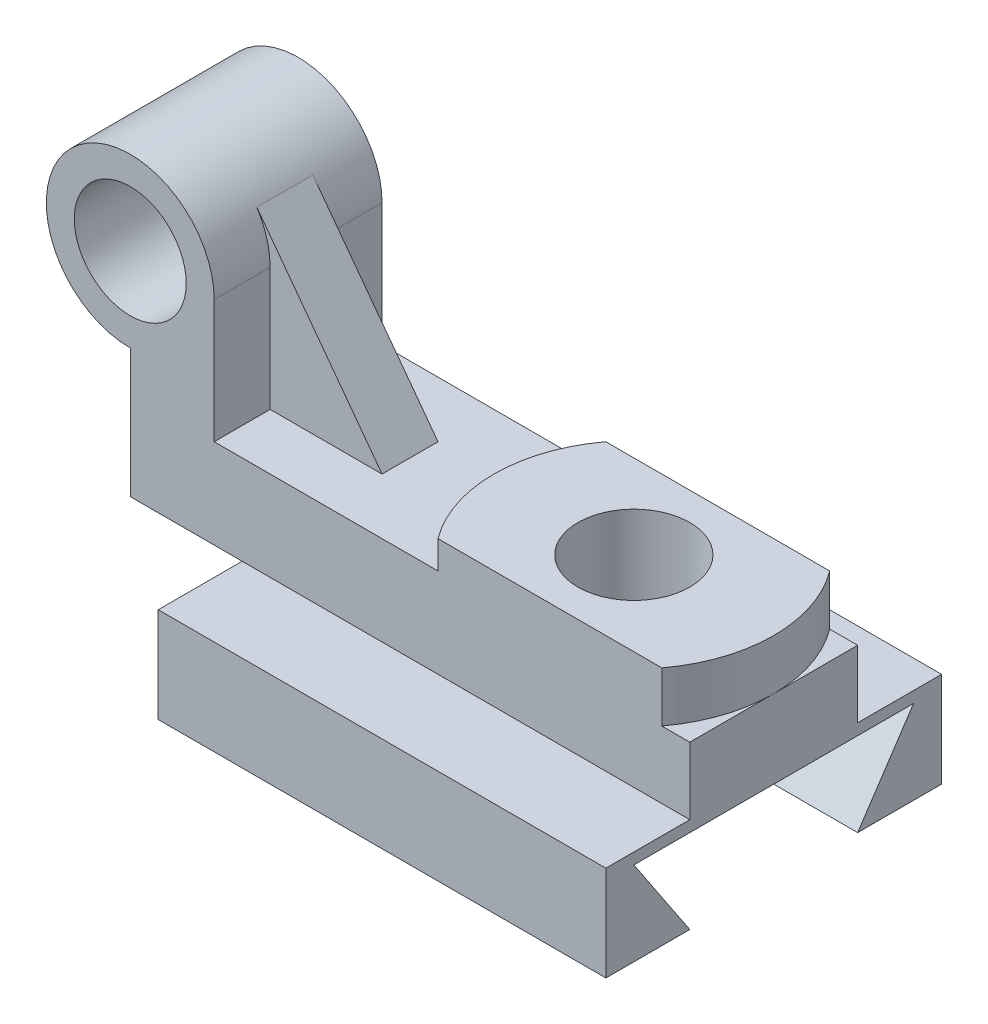
ISO-10303-21;
HEADER;
FILE_DESCRIPTION(('STEP AP214'),'2;1');
FILE_NAME('part.step','',(''),(''),'','','');
FILE_SCHEMA(('AUTOMOTIVE_DESIGN { 1 0 10303 214 1 1 1 1 }'));
ENDSEC;
DATA;
#1=APPLICATION_CONTEXT('core data for automotive mechanical design processes');
#2=APPLICATION_PROTOCOL_DEFINITION('international standard','automotive_design',2000,#1);
#3=PRODUCT_CONTEXT('',#1,'mechanical');
#4=PRODUCT('Part','Part','',(#3));
#5=PRODUCT_RELATED_PRODUCT_CATEGORY('part','',(#4));
#6=PRODUCT_DEFINITION_FORMATION('','',#4);
#7=PRODUCT_DEFINITION_CONTEXT('part definition',#1,'design');
#8=PRODUCT_DEFINITION('design','',#6,#7);
#9=PRODUCT_DEFINITION_SHAPE('','',#8);
#10=(LENGTH_UNIT() NAMED_UNIT(*) SI_UNIT(.MILLI.,.METRE.));
#11=(NAMED_UNIT(*) PLANE_ANGLE_UNIT() SI_UNIT($,.RADIAN.));
#12=(NAMED_UNIT(*) SI_UNIT($,.STERADIAN.) SOLID_ANGLE_UNIT());
#13=UNCERTAINTY_MEASURE_WITH_UNIT(LENGTH_MEASURE(1.E-05),#10,'distance_accuracy_value','');
#14=(GEOMETRIC_REPRESENTATION_CONTEXT(3) GLOBAL_UNCERTAINTY_ASSIGNED_CONTEXT((#13)) GLOBAL_UNIT_ASSIGNED_CONTEXT((#10,
#11,#12)) REPRESENTATION_CONTEXT('',''));
#15=CARTESIAN_POINT('',(0.,0.,0.));
#16=DIRECTION('',(0.,0.,1.));
#17=DIRECTION('',(1.,0.,0.));
#18=AXIS2_PLACEMENT_3D('',#15,#16,#17);
#19=CARTESIAN_POINT('',(-85.,16.,15.));
#20=DIRECTION('',(-1.,0.,0.));
#21=DIRECTION('',(0.,0.,1.));
#22=AXIS2_PLACEMENT_3D('',#19,#20,#21);
#23=PLANE('',#22);
#24=DIRECTION('',(0.,1.,0.));
#25=VECTOR('',#24,1.);
#26=CARTESIAN_POINT('',(-85.,16.,-5.));
#27=LINE('',#26,#25);
#28=CARTESIAN_POINT('',(-85.,16.,-5.));
#29=VERTEX_POINT('',#28);
#30=CARTESIAN_POINT('',(-85.,38.,-5.));
#31=VERTEX_POINT('',#30);
#32=EDGE_CURVE('E197',#29,#31,#27,.T.);
#33=ORIENTED_EDGE('',*,*,#32,.F.);
#34=DIRECTION('',(0.,0.,-1.));
#35=VECTOR('',#34,1.);
#36=CARTESIAN_POINT('',(-85.,16.,15.));
#37=LINE('',#36,#35);
#38=CARTESIAN_POINT('',(-85.,16.,-15.));
#39=VERTEX_POINT('',#38);
#40=EDGE_CURVE('E248',#29,#39,#37,.T.);
#41=ORIENTED_EDGE('',*,*,#40,.T.);
#42=DIRECTION('',(0.,1.,0.));
#43=VECTOR('',#42,1.);
#44=CARTESIAN_POINT('',(-85.,16.,-15.));
#45=LINE('',#44,#43);
#46=CARTESIAN_POINT('',(-85.,38.,-15.));
#47=VERTEX_POINT('',#46);
#48=EDGE_CURVE('E200',#39,#47,#45,.T.);
#49=ORIENTED_EDGE('',*,*,#48,.T.);
#50=DIRECTION('',(0.,0.,-1.));
#51=VECTOR('',#50,1.);
#52=CARTESIAN_POINT('',(-85.,38.,15.));
#53=LINE('',#52,#51);
#54=EDGE_CURVE('E193',#31,#47,#53,.T.);
#55=ORIENTED_EDGE('',*,*,#54,.F.);
#56=EDGE_LOOP('',(#33,#41,#49,#55));
#57=FACE_BOUND('',#56,.T.);
#58=ADVANCED_FACE('F39',(#57),#23,.F.);
#59=CARTESIAN_POINT('',(-25.,21.,0.));
#60=DIRECTION('',(0.,-1.,0.));
#61=DIRECTION('',(0.,0.,-1.));
#62=AXIS2_PLACEMENT_3D('',#59,#60,#61);
#63=CYLINDRICAL_SURFACE('',#62,25.);
#64=CARTESIAN_POINT('',(-25.,16.,0.));
#65=DIRECTION('',(0.,-1.,0.));
#66=DIRECTION('',(0.,0.,-1.));
#67=AXIS2_PLACEMENT_3D('',#64,#65,#66);
#68=CIRCLE('',#67,25.);
#69=CARTESIAN_POINT('',(-45.,16.,15.));
#70=VERTEX_POINT('',#69);
#71=CARTESIAN_POINT('',(-45.,16.,-15.));
#72=VERTEX_POINT('',#71);
#73=EDGE_CURVE('E254',#70,#72,#68,.T.);
#74=ORIENTED_EDGE('',*,*,#73,.F.);
#75=DIRECTION('',(0.,-1.,0.));
#76=VECTOR('',#75,1.);
#77=CARTESIAN_POINT('',(-45.,21.,15.));
#78=LINE('',#77,#76);
#79=CARTESIAN_POINT('',(-45.,21.,15.));
#80=VERTEX_POINT('',#79);
#81=EDGE_CURVE('E268',#70,#80,#78,.F.);
#82=ORIENTED_EDGE('',*,*,#81,.T.);
#83=CARTESIAN_POINT('',(-25.,21.,0.));
#84=DIRECTION('',(0.,1.,0.));
#85=DIRECTION('',(0.,0.,1.));
#86=AXIS2_PLACEMENT_3D('',#83,#84,#85);
#87=CIRCLE('',#86,25.);
#88=CARTESIAN_POINT('',(-45.,21.,-15.));
#89=VERTEX_POINT('',#88);
#90=EDGE_CURVE('E303',#89,#80,#87,.T.);
#91=ORIENTED_EDGE('',*,*,#90,.F.);
#92=DIRECTION('',(0.,-1.,0.));
#93=VECTOR('',#92,1.);
#94=CARTESIAN_POINT('',(-45.,21.,-15.));
#95=LINE('',#94,#93);
#96=EDGE_CURVE('E266',#89,#72,#95,.T.);
#97=ORIENTED_EDGE('',*,*,#96,.T.);
#98=EDGE_LOOP('',(#74,#82,#91,#97));
#99=FACE_BOUND('',#98,.T.);
#100=ADVANCED_FACE('F451',(#99),#63,.T.);
#101=CARTESIAN_POINT('',(-4.99999999999999,21.,15.));
#102=VERTEX_POINT('',#101);
#103=CARTESIAN_POINT('',(-5.,21.,-15.));
#104=VERTEX_POINT('',#103);
#105=EDGE_CURVE('E305',#102,#104,#87,.T.);
#106=ORIENTED_EDGE('',*,*,#105,.F.);
#107=DIRECTION('',(0.,-1.,0.));
#108=VECTOR('',#107,1.);
#109=CARTESIAN_POINT('',(-5.,21.,15.));
#110=LINE('',#109,#108);
#111=CARTESIAN_POINT('',(-4.99999999999999,12.,15.));
#112=VERTEX_POINT('',#111);
#113=EDGE_CURVE('E267',#102,#112,#110,.T.);
#114=ORIENTED_EDGE('',*,*,#113,.T.);
#115=CARTESIAN_POINT('',(-25.,12.,0.));
#116=DIRECTION('',(0.,1.,0.));
#117=DIRECTION('',(0.,0.,1.));
#118=AXIS2_PLACEMENT_3D('',#115,#116,#117);
#119=CIRCLE('',#118,25.);
#120=CARTESIAN_POINT('',(0.,12.,0.));
#121=VERTEX_POINT('',#120);
#122=EDGE_CURVE('E50',#112,#121,#119,.T.);
#123=ORIENTED_EDGE('',*,*,#122,.T.);
#124=CARTESIAN_POINT('',(-5.,12.,-15.));
#125=VERTEX_POINT('',#124);
#126=EDGE_CURVE('E363',#121,#125,#119,.T.);
#127=ORIENTED_EDGE('',*,*,#126,.T.);
#128=DIRECTION('',(0.,-1.,0.));
#129=VECTOR('',#128,1.);
#130=CARTESIAN_POINT('',(-5.,21.,-15.));
#131=LINE('',#130,#129);
#132=EDGE_CURVE('E265',#125,#104,#131,.F.);
#133=ORIENTED_EDGE('',*,*,#132,.T.);
#134=EDGE_LOOP('',(#106,#114,#123,#127,#133));
#135=FACE_BOUND('',#134,.T.);
#136=ADVANCED_FACE('F377',(#135),#63,.T.);
#137=CARTESIAN_POINT('',(-80.,0.,-30.));
#138=DIRECTION('',(0.,1.,0.));
#139=DIRECTION('',(0.,0.,1.));
#140=AXIS2_PLACEMENT_3D('',#137,#138,#139);
#141=PLANE('',#140);
#142=DIRECTION('',(1.,0.,0.));
#143=VECTOR('',#142,1.);
#144=CARTESIAN_POINT('',(-100.,0.,15.));
#145=LINE('',#144,#143);
#146=CARTESIAN_POINT('',(-80.,0.,15.));
#147=VERTEX_POINT('',#146);
#148=CARTESIAN_POINT('',(0.,0.,15.));
#149=VERTEX_POINT('',#148);
#150=EDGE_CURVE('E285',#147,#149,#145,.T.);
#151=ORIENTED_EDGE('',*,*,#150,.F.);
#152=DIRECTION('',(0.,0.,1.));
#153=VECTOR('',#152,1.);
#154=CARTESIAN_POINT('',(-80.,0.,-30.));
#155=LINE('',#154,#153);
#156=CARTESIAN_POINT('',(-80.,0.,30.));
#157=VERTEX_POINT('',#156);
#158=EDGE_CURVE('E329',#147,#157,#155,.T.);
#159=ORIENTED_EDGE('',*,*,#158,.T.);
#160=DIRECTION('',(1.,0.,0.));
#161=VECTOR('',#160,1.);
#162=CARTESIAN_POINT('',(-80.,0.,30.));
#163=LINE('',#162,#161);
#164=CARTESIAN_POINT('',(0.,0.,30.));
#165=VERTEX_POINT('',#164);
#166=EDGE_CURVE('E359',#157,#165,#163,.T.);
#167=ORIENTED_EDGE('',*,*,#166,.T.);
#168=DIRECTION('',(0.,0.,1.));
#169=VECTOR('',#168,1.);
#170=CARTESIAN_POINT('',(0.,0.,-30.));
#171=LINE('',#170,#169);
#172=EDGE_CURVE('E354',#149,#165,#171,.T.);
#173=ORIENTED_EDGE('',*,*,#172,.F.);
#174=EDGE_LOOP('',(#151,#159,#167,#173));
#175=FACE_BOUND('',#174,.T.);
#176=ADVANCED_FACE('F394',(#175),#141,.T.);
#177=CARTESIAN_POINT('',(-80.,0.,30.));
#178=DIRECTION('',(0.,0.,1.));
#179=DIRECTION('',(0.,-1.,0.));
#180=AXIS2_PLACEMENT_3D('',#177,#178,#179);
#181=PLANE('',#180);
#182=DIRECTION('',(0.,-1.,0.));
#183=VECTOR('',#182,1.);
#184=CARTESIAN_POINT('',(0.,0.,30.));
#185=LINE('',#184,#183);
#186=CARTESIAN_POINT('',(0.,-17.,30.));
#187=VERTEX_POINT('',#186);
#188=EDGE_CURVE('E306',#165,#187,#185,.T.);
#189=ORIENTED_EDGE('',*,*,#188,.F.);
#190=ORIENTED_EDGE('',*,*,#166,.F.);
#191=DIRECTION('',(0.,-1.,0.));
#192=VECTOR('',#191,1.);
#193=CARTESIAN_POINT('',(-80.,0.,30.));
#194=LINE('',#193,#192);
#195=CARTESIAN_POINT('',(-80.,-17.,30.));
#196=VERTEX_POINT('',#195);
#197=EDGE_CURVE('E310',#157,#196,#194,.T.);
#198=ORIENTED_EDGE('',*,*,#197,.T.);
#199=DIRECTION('',(1.,0.,0.));
#200=VECTOR('',#199,1.);
#201=CARTESIAN_POINT('',(-80.,-17.,30.));
#202=LINE('',#201,#200);
#203=EDGE_CURVE('E331',#196,#187,#202,.T.);
#204=ORIENTED_EDGE('',*,*,#203,.T.);
#205=EDGE_LOOP('',(#189,#190,#198,#204));
#206=FACE_BOUND('',#205,.T.);
#207=ADVANCED_FACE('F41',(#206),#181,.T.);
#208=DIRECTION('',(1.,0.,0.));
#209=VECTOR('',#208,1.);
#210=CARTESIAN_POINT('',(-100.,0.,-15.));
#211=LINE('',#210,#209);
#212=CARTESIAN_POINT('',(-80.,0.,-15.));
#213=VERTEX_POINT('',#212);
#214=CARTESIAN_POINT('',(0.,0.,-15.));
#215=VERTEX_POINT('',#214);
#216=EDGE_CURVE('E297',#213,#215,#211,.T.);
#217=ORIENTED_EDGE('',*,*,#216,.T.);
#218=CARTESIAN_POINT('',(0.,0.,-30.));
#219=VERTEX_POINT('',#218);
#220=EDGE_CURVE('E311',#219,#215,#171,.T.);
#221=ORIENTED_EDGE('',*,*,#220,.F.);
#222=DIRECTION('',(1.,0.,0.));
#223=VECTOR('',#222,1.);
#224=CARTESIAN_POINT('',(-80.,0.,-30.));
#225=LINE('',#224,#223);
#226=CARTESIAN_POINT('',(-80.,0.,-30.));
#227=VERTEX_POINT('',#226);
#228=EDGE_CURVE('E362',#227,#219,#225,.T.);
#229=ORIENTED_EDGE('',*,*,#228,.F.);
#230=EDGE_CURVE('E332',#227,#213,#155,.T.);
#231=ORIENTED_EDGE('',*,*,#230,.T.);
#232=EDGE_LOOP('',(#217,#221,#229,#231));
#233=FACE_BOUND('',#232,.T.);
#234=ADVANCED_FACE('F428',(#233),#141,.T.);
#235=CARTESIAN_POINT('',(-80.,-17.,-30.));
#236=DIRECTION('',(0.,0.,-1.));
#237=DIRECTION('',(0.,1.,0.));
#238=AXIS2_PLACEMENT_3D('',#235,#236,#237);
#239=PLANE('',#238);
#240=DIRECTION('',(0.,1.,0.));
#241=VECTOR('',#240,1.);
#242=CARTESIAN_POINT('',(0.,-17.,-30.));
#243=LINE('',#242,#241);
#244=CARTESIAN_POINT('',(0.,-17.,-30.));
#245=VERTEX_POINT('',#244);
#246=EDGE_CURVE('E355',#245,#219,#243,.T.);
#247=ORIENTED_EDGE('',*,*,#246,.F.);
#248=DIRECTION('',(1.,0.,0.));
#249=VECTOR('',#248,1.);
#250=CARTESIAN_POINT('',(-80.,-17.,-30.));
#251=LINE('',#250,#249);
#252=CARTESIAN_POINT('',(-80.,-17.,-30.));
#253=VERTEX_POINT('',#252);
#254=EDGE_CURVE('E365',#253,#245,#251,.T.);
#255=ORIENTED_EDGE('',*,*,#254,.F.);
#256=DIRECTION('',(0.,1.,0.));
#257=VECTOR('',#256,1.);
#258=CARTESIAN_POINT('',(-80.,-17.,-30.));
#259=LINE('',#258,#257);
#260=EDGE_CURVE('E330',#253,#227,#259,.T.);
#261=ORIENTED_EDGE('',*,*,#260,.T.);
#262=ORIENTED_EDGE('',*,*,#228,.T.);
#263=EDGE_LOOP('',(#247,#255,#261,#262));
#264=FACE_BOUND('',#263,.T.);
#265=ADVANCED_FACE('F422',(#264),#239,.T.);
#266=CARTESIAN_POINT('',(-80.,-17.,-15.));
#267=DIRECTION('',(0.,-1.,0.));
#268=DIRECTION('',(0.,0.,-1.));
#269=AXIS2_PLACEMENT_3D('',#266,#267,#268);
#270=PLANE('',#269);
#271=DIRECTION('',(0.,0.,-1.));
#272=VECTOR('',#271,1.);
#273=CARTESIAN_POINT('',(0.,-17.,-15.));
#274=LINE('',#273,#272);
#275=CARTESIAN_POINT('',(0.,-17.,-15.));
#276=VERTEX_POINT('',#275);
#277=EDGE_CURVE('E349',#276,#245,#274,.T.);
#278=ORIENTED_EDGE('',*,*,#277,.F.);
#279=DIRECTION('',(1.,0.,0.));
#280=VECTOR('',#279,1.);
#281=CARTESIAN_POINT('',(-80.,-17.,-15.));
#282=LINE('',#281,#280);
#283=CARTESIAN_POINT('',(-80.,-17.,-15.));
#284=VERTEX_POINT('',#283);
#285=EDGE_CURVE('E368',#284,#276,#282,.T.);
#286=ORIENTED_EDGE('',*,*,#285,.F.);
#287=DIRECTION('',(0.,0.,-1.));
#288=VECTOR('',#287,1.);
#289=CARTESIAN_POINT('',(-80.,-17.,-15.));
#290=LINE('',#289,#288);
#291=EDGE_CURVE('E322',#284,#253,#290,.T.);
#292=ORIENTED_EDGE('',*,*,#291,.T.);
#293=ORIENTED_EDGE('',*,*,#254,.T.);
#294=EDGE_LOOP('',(#278,#286,#292,#293));
#295=FACE_BOUND('',#294,.T.);
#296=ADVANCED_FACE('F423',(#295),#270,.T.);
#297=CARTESIAN_POINT('',(-80.,-2.00000000000001,-25.));
#298=DIRECTION('',(0.,0.554700196225229,0.832050294337844));
#299=DIRECTION('',(0.,-0.832050294337844,0.554700196225229));
#300=AXIS2_PLACEMENT_3D('',#297,#298,#299);
#301=PLANE('',#300);
#302=DIRECTION('',(0.,-0.832050294337844,0.554700196225229));
#303=VECTOR('',#302,1.);
#304=CARTESIAN_POINT('',(0.,-2.00000000000001,-25.));
#305=LINE('',#304,#303);
#306=CARTESIAN_POINT('',(0.,-2.00000000000001,-25.));
#307=VERTEX_POINT('',#306);
#308=EDGE_CURVE('E347',#307,#276,#305,.T.);
#309=ORIENTED_EDGE('',*,*,#308,.F.);
#310=DIRECTION('',(1.,0.,0.));
#311=VECTOR('',#310,1.);
#312=CARTESIAN_POINT('',(-80.,-2.00000000000001,-25.));
#313=LINE('',#312,#311);
#314=CARTESIAN_POINT('',(-80.,-2.00000000000001,-25.));
#315=VERTEX_POINT('',#314);
#316=EDGE_CURVE('E366',#315,#307,#313,.T.);
#317=ORIENTED_EDGE('',*,*,#316,.F.);
#318=DIRECTION('',(0.,-0.832050294337844,0.554700196225229));
#319=VECTOR('',#318,1.);
#320=CARTESIAN_POINT('',(-80.,-2.00000000000001,-25.));
#321=LINE('',#320,#319);
#322=EDGE_CURVE('E321',#315,#284,#321,.T.);
#323=ORIENTED_EDGE('',*,*,#322,.T.);
#324=ORIENTED_EDGE('',*,*,#285,.T.);
#325=EDGE_LOOP('',(#309,#317,#323,#324));
#326=FACE_BOUND('',#325,.T.);
#327=ADVANCED_FACE('F417',(#326),#301,.T.);
#328=CARTESIAN_POINT('',(-80.,-2.00000000000001,25.));
#329=DIRECTION('',(0.,-1.,0.));
#330=DIRECTION('',(0.,0.,-1.));
#331=AXIS2_PLACEMENT_3D('',#328,#329,#330);
#332=PLANE('',#331);
#333=CARTESIAN_POINT('',(-25.,-2.00000000000001,0.));
#334=DIRECTION('',(0.,-1.,0.));
#335=DIRECTION('',(0.,0.,-1.));
#336=AXIS2_PLACEMENT_3D('',#333,#334,#335);
#337=CIRCLE('',#336,10.);
#338=CARTESIAN_POINT('',(-25.,-2.00000000000001,-10.));
#339=VERTEX_POINT('',#338);
#340=EDGE_CURVE('E485',#339,#339,#337,.T.);
#341=ORIENTED_EDGE('',*,*,#340,.F.);
#342=EDGE_LOOP('',(#341));
#343=FACE_BOUND('',#342,.T.);
#344=DIRECTION('',(0.,0.,-1.));
#345=VECTOR('',#344,1.);
#346=CARTESIAN_POINT('',(-80.,-2.00000000000001,25.));
#347=LINE('',#346,#345);
#348=CARTESIAN_POINT('',(-80.,-2.00000000000001,25.));
#349=VERTEX_POINT('',#348);
#350=EDGE_CURVE('E317',#349,#315,#347,.T.);
#351=ORIENTED_EDGE('',*,*,#350,.T.);
#352=ORIENTED_EDGE('',*,*,#316,.T.);
#353=DIRECTION('',(0.,0.,-1.));
#354=VECTOR('',#353,1.);
#355=CARTESIAN_POINT('',(0.,-2.00000000000001,25.));
#356=LINE('',#355,#354);
#357=CARTESIAN_POINT('',(0.,-2.00000000000001,25.));
#358=VERTEX_POINT('',#357);
#359=EDGE_CURVE('E344',#358,#307,#356,.T.);
#360=ORIENTED_EDGE('',*,*,#359,.F.);
#361=DIRECTION('',(1.,0.,0.));
#362=VECTOR('',#361,1.);
#363=CARTESIAN_POINT('',(-80.,-2.00000000000001,25.));
#364=LINE('',#363,#362);
#365=EDGE_CURVE('E367',#349,#358,#364,.T.);
#366=ORIENTED_EDGE('',*,*,#365,.F.);
#367=EDGE_LOOP('',(#351,#352,#360,#366));
#368=FACE_BOUND('',#367,.T.);
#369=ADVANCED_FACE('F412',(#343,#368),#332,.T.);
#370=CARTESIAN_POINT('',(-80.,-17.,15.));
#371=DIRECTION('',(0.,0.554700196225229,-0.832050294337844));
#372=DIRECTION('',(0.,0.832050294337844,0.554700196225229));
#373=AXIS2_PLACEMENT_3D('',#370,#371,#372);
#374=PLANE('',#373);
#375=DIRECTION('',(0.,0.832050294337844,0.554700196225229));
#376=VECTOR('',#375,1.);
#377=CARTESIAN_POINT('',(0.,-17.,15.));
#378=LINE('',#377,#376);
#379=CARTESIAN_POINT('',(0.,-17.,15.));
#380=VERTEX_POINT('',#379);
#381=EDGE_CURVE('E339',#380,#358,#378,.T.);
#382=ORIENTED_EDGE('',*,*,#381,.F.);
#383=DIRECTION('',(1.,0.,0.));
#384=VECTOR('',#383,1.);
#385=CARTESIAN_POINT('',(-80.,-17.,15.));
#386=LINE('',#385,#384);
#387=CARTESIAN_POINT('',(-80.,-17.,15.));
#388=VERTEX_POINT('',#387);
#389=EDGE_CURVE('E375',#388,#380,#386,.T.);
#390=ORIENTED_EDGE('',*,*,#389,.F.);
#391=DIRECTION('',(0.,0.832050294337844,0.554700196225229));
#392=VECTOR('',#391,1.);
#393=CARTESIAN_POINT('',(-80.,-17.,15.));
#394=LINE('',#393,#392);
#395=EDGE_CURVE('E316',#388,#349,#394,.T.);
#396=ORIENTED_EDGE('',*,*,#395,.T.);
#397=ORIENTED_EDGE('',*,*,#365,.T.);
#398=EDGE_LOOP('',(#382,#390,#396,#397));
#399=FACE_BOUND('',#398,.T.);
#400=ADVANCED_FACE('F406',(#399),#374,.T.);
#401=CARTESIAN_POINT('',(-80.,-17.,30.));
#402=DIRECTION('',(0.,-1.,0.));
#403=DIRECTION('',(0.,0.,-1.));
#404=AXIS2_PLACEMENT_3D('',#401,#402,#403);
#405=PLANE('',#404);
#406=DIRECTION('',(0.,0.,-1.));
#407=VECTOR('',#406,1.);
#408=CARTESIAN_POINT('',(0.,-17.,30.));
#409=LINE('',#408,#407);
#410=EDGE_CURVE('E340',#187,#380,#409,.T.);
#411=ORIENTED_EDGE('',*,*,#410,.F.);
#412=ORIENTED_EDGE('',*,*,#203,.F.);
#413=DIRECTION('',(0.,0.,-1.));
#414=VECTOR('',#413,1.);
#415=CARTESIAN_POINT('',(-80.,-17.,30.));
#416=LINE('',#415,#414);
#417=EDGE_CURVE('E315',#196,#388,#416,.T.);
#418=ORIENTED_EDGE('',*,*,#417,.T.);
#419=ORIENTED_EDGE('',*,*,#389,.T.);
#420=EDGE_LOOP('',(#411,#412,#418,#419));
#421=FACE_BOUND('',#420,.T.);
#422=ADVANCED_FACE('F404',(#421),#405,.T.);
#423=CARTESIAN_POINT('',(-80.,0.,0.));
#424=DIRECTION('',(1.,0.,0.));
#425=DIRECTION('',(0.,0.,-1.));
#426=AXIS2_PLACEMENT_3D('',#423,#424,#425);
#427=PLANE('',#426);
#428=DIRECTION('',(0.,0.,-1.));
#429=VECTOR('',#428,1.);
#430=CARTESIAN_POINT('',(-80.,0.,0.));
#431=LINE('',#430,#429);
#432=EDGE_CURVE('E291',#147,#213,#431,.T.);
#433=ORIENTED_EDGE('',*,*,#432,.T.);
#434=ORIENTED_EDGE('',*,*,#230,.F.);
#435=ORIENTED_EDGE('',*,*,#260,.F.);
#436=ORIENTED_EDGE('',*,*,#291,.F.);
#437=ORIENTED_EDGE('',*,*,#322,.F.);
#438=ORIENTED_EDGE('',*,*,#350,.F.);
#439=ORIENTED_EDGE('',*,*,#395,.F.);
#440=ORIENTED_EDGE('',*,*,#417,.F.);
#441=ORIENTED_EDGE('',*,*,#197,.F.);
#442=ORIENTED_EDGE('',*,*,#158,.F.);
#443=EDGE_LOOP('',(#433,#434,#435,#436,#437,#438,#439,#440,#441,#442));
#444=FACE_BOUND('',#443,.T.);
#445=ADVANCED_FACE('F512',(#444),#427,.F.);
#446=CARTESIAN_POINT('',(0.,0.,0.));
#447=DIRECTION('',(1.,0.,0.));
#448=DIRECTION('',(0.,0.,-1.));
#449=AXIS2_PLACEMENT_3D('',#446,#447,#448);
#450=PLANE('',#449);
#451=DIRECTION('',(0.,-1.,0.));
#452=VECTOR('',#451,1.);
#453=CARTESIAN_POINT('',(0.,0.,15.));
#454=LINE('',#453,#452);
#455=CARTESIAN_POINT('',(0.,12.,15.));
#456=VERTEX_POINT('',#455);
#457=EDGE_CURVE('E271',#456,#149,#454,.T.);
#458=ORIENTED_EDGE('',*,*,#457,.T.);
#459=ORIENTED_EDGE('',*,*,#172,.T.);
#460=ORIENTED_EDGE('',*,*,#188,.T.);
#461=ORIENTED_EDGE('',*,*,#410,.T.);
#462=ORIENTED_EDGE('',*,*,#381,.T.);
#463=ORIENTED_EDGE('',*,*,#359,.T.);
#464=ORIENTED_EDGE('',*,*,#308,.T.);
#465=ORIENTED_EDGE('',*,*,#277,.T.);
#466=ORIENTED_EDGE('',*,*,#246,.T.);
#467=ORIENTED_EDGE('',*,*,#220,.T.);
#468=DIRECTION('',(0.,1.,0.));
#469=VECTOR('',#468,1.);
#470=CARTESIAN_POINT('',(0.,0.,-15.));
#471=LINE('',#470,#469);
#472=CARTESIAN_POINT('',(0.,12.,-15.));
#473=VERTEX_POINT('',#472);
#474=EDGE_CURVE('E284',#215,#473,#471,.T.);
#475=ORIENTED_EDGE('',*,*,#474,.T.);
#476=DIRECTION('',(0.,0.,1.));
#477=VECTOR('',#476,1.);
#478=CARTESIAN_POINT('',(0.,12.,15.));
#479=LINE('',#478,#477);
#480=EDGE_CURVE('E280',#473,#121,#479,.T.);
#481=ORIENTED_EDGE('',*,*,#480,.T.);
#482=EDGE_CURVE('E289',#121,#456,#479,.T.);
#483=ORIENTED_EDGE('',*,*,#482,.T.);
#484=EDGE_LOOP('',(#458,#459,#460,#461,#462,#463,#464,#465,#466,#467,#475,#481,#483));
#485=FACE_BOUND('',#484,.T.);
#486=ADVANCED_FACE('F391',(#485),#450,.T.);
#487=CARTESIAN_POINT('',(-25.,21.,0.));
#488=DIRECTION('',(0.,1.,0.));
#489=DIRECTION('',(0.,0.,1.));
#490=AXIS2_PLACEMENT_3D('',#487,#488,#489);
#491=PLANE('',#490);
#492=CARTESIAN_POINT('',(-25.,21.,0.));
#493=DIRECTION('',(0.,1.,0.));
#494=DIRECTION('',(0.,0.,1.));
#495=AXIS2_PLACEMENT_3D('',#492,#493,#494);
#496=CIRCLE('',#495,10.);
#497=CARTESIAN_POINT('',(-25.,21.,10.));
#498=VERTEX_POINT('',#497);
#499=EDGE_CURVE('E482',#498,#498,#496,.T.);
#500=ORIENTED_EDGE('',*,*,#499,.F.);
#501=EDGE_LOOP('',(#500));
#502=FACE_BOUND('',#501,.T.);
#503=DIRECTION('',(1.,0.,0.));
#504=VECTOR('',#503,1.);
#505=CARTESIAN_POINT('',(-100.,21.,15.));
#506=LINE('',#505,#504);
#507=EDGE_CURVE('E259',#80,#102,#506,.T.);
#508=ORIENTED_EDGE('',*,*,#507,.T.);
#509=ORIENTED_EDGE('',*,*,#105,.T.);
#510=DIRECTION('',(1.,0.,0.));
#511=VECTOR('',#510,1.);
#512=CARTESIAN_POINT('',(-100.,21.,-15.));
#513=LINE('',#512,#511);
#514=EDGE_CURVE('E256',#89,#104,#513,.T.);
#515=ORIENTED_EDGE('',*,*,#514,.F.);
#516=ORIENTED_EDGE('',*,*,#90,.T.);
#517=EDGE_LOOP('',(#508,#509,#515,#516));
#518=FACE_BOUND('',#517,.T.);
#519=ADVANCED_FACE('F493',(#502,#518),#491,.T.);
#520=CARTESIAN_POINT('',(-100.,0.,0.));
#521=DIRECTION('',(-1.,0.,0.));
#522=DIRECTION('',(0.,0.,1.));
#523=AXIS2_PLACEMENT_3D('',#520,#521,#522);
#524=PLANE('',#523);
#525=DIRECTION('',(0.,0.,-1.));
#526=VECTOR('',#525,1.);
#527=CARTESIAN_POINT('',(-100.,23.,15.));
#528=LINE('',#527,#526);
#529=CARTESIAN_POINT('',(-100.,23.,15.));
#530=VERTEX_POINT('',#529);
#531=CARTESIAN_POINT('',(-100.,23.,-15.));
#532=VERTEX_POINT('',#531);
#533=EDGE_CURVE('E251',#530,#532,#528,.T.);
#534=ORIENTED_EDGE('',*,*,#533,.T.);
#535=DIRECTION('',(0.,1.,0.));
#536=VECTOR('',#535,1.);
#537=CARTESIAN_POINT('',(-100.,0.,-15.));
#538=LINE('',#537,#536);
#539=CARTESIAN_POINT('',(-100.,0.,-15.));
#540=VERTEX_POINT('',#539);
#541=EDGE_CURVE('E276',#540,#532,#538,.T.);
#542=ORIENTED_EDGE('',*,*,#541,.F.);
#543=DIRECTION('',(0.,0.,-1.));
#544=VECTOR('',#543,1.);
#545=CARTESIAN_POINT('',(-100.,0.,15.));
#546=LINE('',#545,#544);
#547=CARTESIAN_POINT('',(-100.,0.,15.));
#548=VERTEX_POINT('',#547);
#549=EDGE_CURVE('E277',#548,#540,#546,.T.);
#550=ORIENTED_EDGE('',*,*,#549,.F.);
#551=DIRECTION('',(0.,-1.,0.));
#552=VECTOR('',#551,1.);
#553=CARTESIAN_POINT('',(-100.,0.,15.));
#554=LINE('',#553,#552);
#555=EDGE_CURVE('E272',#530,#548,#554,.T.);
#556=ORIENTED_EDGE('',*,*,#555,.F.);
#557=EDGE_LOOP('',(#534,#542,#550,#556));
#558=FACE_BOUND('',#557,.T.);
#559=ADVANCED_FACE('F500',(#558),#524,.T.);
#560=CARTESIAN_POINT('',(-100.,0.,15.));
#561=DIRECTION('',(0.,-1.,0.));
#562=DIRECTION('',(0.,0.,-1.));
#563=AXIS2_PLACEMENT_3D('',#560,#561,#562);
#564=PLANE('',#563);
#565=ORIENTED_EDGE('',*,*,#549,.T.);
#566=EDGE_CURVE('E298',#540,#213,#211,.T.);
#567=ORIENTED_EDGE('',*,*,#566,.T.);
#568=ORIENTED_EDGE('',*,*,#432,.F.);
#569=EDGE_CURVE('E299',#548,#147,#145,.T.);
#570=ORIENTED_EDGE('',*,*,#569,.F.);
#571=EDGE_LOOP('',(#565,#567,#568,#570));
#572=FACE_BOUND('',#571,.T.);
#573=ADVANCED_FACE('F508',(#572),#564,.T.);
#574=CARTESIAN_POINT('',(-100.,0.,15.));
#575=DIRECTION('',(0.,0.,1.));
#576=DIRECTION('',(1.,0.,0.));
#577=AXIS2_PLACEMENT_3D('',#574,#575,#576);
#578=PLANE('',#577);
#579=ORIENTED_EDGE('',*,*,#150,.T.);
#580=ORIENTED_EDGE('',*,*,#457,.F.);
#581=DIRECTION('',(1.,0.,0.));
#582=VECTOR('',#581,1.);
#583=CARTESIAN_POINT('',(-100.,12.,15.));
#584=LINE('',#583,#582);
#585=EDGE_CURVE('E292',#112,#456,#584,.T.);
#586=ORIENTED_EDGE('',*,*,#585,.F.);
#587=ORIENTED_EDGE('',*,*,#113,.F.);
#588=ORIENTED_EDGE('',*,*,#507,.F.);
#589=ORIENTED_EDGE('',*,*,#81,.F.);
#590=DIRECTION('',(-1.,0.,0.));
#591=VECTOR('',#590,1.);
#592=CARTESIAN_POINT('',(-45.,16.,15.));
#593=LINE('',#592,#591);
#594=CARTESIAN_POINT('',(-85.,16.,15.));
#595=VERTEX_POINT('',#594);
#596=EDGE_CURVE('E238',#70,#595,#593,.T.);
#597=ORIENTED_EDGE('',*,*,#596,.T.);
#598=DIRECTION('',(0.,1.,0.));
#599=VECTOR('',#598,1.);
#600=CARTESIAN_POINT('',(-85.,16.,15.));
#601=LINE('',#600,#599);
#602=CARTESIAN_POINT('',(-85.,38.,15.));
#603=VERTEX_POINT('',#602);
#604=EDGE_CURVE('E204',#595,#603,#601,.T.);
#605=ORIENTED_EDGE('',*,*,#604,.T.);
#606=CARTESIAN_POINT('',(-100.,38.,15.));
#607=DIRECTION('',(0.,0.,1.));
#608=DIRECTION('',(1.,0.,0.));
#609=AXIS2_PLACEMENT_3D('',#606,#607,#608);
#610=CIRCLE('',#609,15.);
#611=EDGE_CURVE('E240',#603,#530,#610,.T.);
#612=ORIENTED_EDGE('',*,*,#611,.T.);
#613=ORIENTED_EDGE('',*,*,#555,.T.);
#614=ORIENTED_EDGE('',*,*,#569,.T.);
#615=EDGE_LOOP('',(#579,#580,#586,#587,#588,#589,#597,#605,#612,#613,#614));
#616=FACE_BOUND('',#615,.T.);
#617=CARTESIAN_POINT('',(-100.,38.,15.));
#618=DIRECTION('',(0.,0.,1.));
#619=DIRECTION('',(1.,0.,0.));
#620=AXIS2_PLACEMENT_3D('',#617,#618,#619);
#621=CIRCLE('',#620,9.99999999999999);
#622=CARTESIAN_POINT('',(-90.,38.,15.));
#623=VERTEX_POINT('',#622);
#624=EDGE_CURVE('E231',#623,#623,#621,.T.);
#625=ORIENTED_EDGE('',*,*,#624,.F.);
#626=EDGE_LOOP('',(#625));
#627=FACE_BOUND('',#626,.T.);
#628=ADVANCED_FACE('F390',(#616,#627),#578,.T.);
#629=CARTESIAN_POINT('',(-100.,12.,15.));
#630=DIRECTION('',(0.,1.,0.));
#631=DIRECTION('',(0.,0.,1.));
#632=AXIS2_PLACEMENT_3D('',#629,#630,#631);
#633=PLANE('',#632);
#634=ORIENTED_EDGE('',*,*,#122,.F.);
#635=ORIENTED_EDGE('',*,*,#585,.T.);
#636=ORIENTED_EDGE('',*,*,#482,.F.);
#637=EDGE_LOOP('',(#634,#635,#636));
#638=FACE_BOUND('',#637,.T.);
#639=ADVANCED_FACE('F382',(#638),#633,.T.);
#640=ORIENTED_EDGE('',*,*,#126,.F.);
#641=ORIENTED_EDGE('',*,*,#480,.F.);
#642=DIRECTION('',(1.,0.,0.));
#643=VECTOR('',#642,1.);
#644=CARTESIAN_POINT('',(-100.,12.,-15.));
#645=LINE('',#644,#643);
#646=EDGE_CURVE('E294',#125,#473,#645,.T.);
#647=ORIENTED_EDGE('',*,*,#646,.F.);
#648=EDGE_LOOP('',(#640,#641,#647));
#649=FACE_BOUND('',#648,.T.);
#650=ADVANCED_FACE('F438',(#649),#633,.T.);
#651=CARTESIAN_POINT('',(-100.,0.,-15.));
#652=DIRECTION('',(0.,0.,-1.));
#653=DIRECTION('',(-1.,0.,0.));
#654=AXIS2_PLACEMENT_3D('',#651,#652,#653);
#655=PLANE('',#654);
#656=ORIENTED_EDGE('',*,*,#474,.F.);
#657=ORIENTED_EDGE('',*,*,#216,.F.);
#658=ORIENTED_EDGE('',*,*,#566,.F.);
#659=ORIENTED_EDGE('',*,*,#541,.T.);
#660=CARTESIAN_POINT('',(-100.,38.,-15.));
#661=DIRECTION('',(0.,0.,1.));
#662=DIRECTION('',(1.,0.,0.));
#663=AXIS2_PLACEMENT_3D('',#660,#661,#662);
#664=CIRCLE('',#663,15.);
#665=EDGE_CURVE('E233',#47,#532,#664,.T.);
#666=ORIENTED_EDGE('',*,*,#665,.F.);
#667=ORIENTED_EDGE('',*,*,#48,.F.);
#668=DIRECTION('',(-1.,0.,0.));
#669=VECTOR('',#668,1.);
#670=CARTESIAN_POINT('',(-45.,16.,-15.));
#671=LINE('',#670,#669);
#672=EDGE_CURVE('E242',#72,#39,#671,.T.);
#673=ORIENTED_EDGE('',*,*,#672,.F.);
#674=ORIENTED_EDGE('',*,*,#96,.F.);
#675=ORIENTED_EDGE('',*,*,#514,.T.);
#676=ORIENTED_EDGE('',*,*,#132,.F.);
#677=ORIENTED_EDGE('',*,*,#646,.T.);
#678=EDGE_LOOP('',(#656,#657,#658,#659,#666,#667,#673,#674,#675,#676,#677));
#679=FACE_BOUND('',#678,.T.);
#680=CARTESIAN_POINT('',(-100.,38.,-15.));
#681=DIRECTION('',(0.,0.,1.));
#682=DIRECTION('',(1.,0.,0.));
#683=AXIS2_PLACEMENT_3D('',#680,#681,#682);
#684=CIRCLE('',#683,9.99999999999999);
#685=CARTESIAN_POINT('',(-90.,38.,-15.));
#686=VERTEX_POINT('',#685);
#687=EDGE_CURVE('E229',#686,#686,#684,.T.);
#688=ORIENTED_EDGE('',*,*,#687,.T.);
#689=EDGE_LOOP('',(#688));
#690=FACE_BOUND('',#689,.T.);
#691=ADVANCED_FACE('F432',(#679,#690),#655,.T.);
#692=CARTESIAN_POINT('',(-45.,16.,15.));
#693=DIRECTION('',(0.,-1.,0.));
#694=DIRECTION('',(0.,0.,-1.));
#695=AXIS2_PLACEMENT_3D('',#692,#693,#694);
#696=PLANE('',#695);
#697=DIRECTION('',(0.,0.,-1.));
#698=VECTOR('',#697,1.);
#699=CARTESIAN_POINT('',(-65.,16.,15.));
#700=LINE('',#699,#698);
#701=CARTESIAN_POINT('',(-65.,16.,-5.));
#702=VERTEX_POINT('',#701);
#703=CARTESIAN_POINT('',(-65.,16.,5.));
#704=VERTEX_POINT('',#703);
#705=EDGE_CURVE('E53',#702,#704,#700,.F.);
#706=ORIENTED_EDGE('',*,*,#705,.T.);
#707=DIRECTION('',(-1.,0.,0.));
#708=VECTOR('',#707,1.);
#709=CARTESIAN_POINT('',(-45.,16.,5.));
#710=LINE('',#709,#708);
#711=CARTESIAN_POINT('',(-85.,16.,5.));
#712=VERTEX_POINT('',#711);
#713=EDGE_CURVE('E230',#704,#712,#710,.T.);
#714=ORIENTED_EDGE('',*,*,#713,.T.);
#715=EDGE_CURVE('E250',#595,#712,#37,.T.);
#716=ORIENTED_EDGE('',*,*,#715,.F.);
#717=ORIENTED_EDGE('',*,*,#596,.F.);
#718=ORIENTED_EDGE('',*,*,#73,.T.);
#719=ORIENTED_EDGE('',*,*,#672,.T.);
#720=ORIENTED_EDGE('',*,*,#40,.F.);
#721=DIRECTION('',(-1.,0.,0.));
#722=VECTOR('',#721,1.);
#723=CARTESIAN_POINT('',(-45.,16.,-5.));
#724=LINE('',#723,#722);
#725=EDGE_CURVE('E56',#702,#29,#724,.T.);
#726=ORIENTED_EDGE('',*,*,#725,.F.);
#727=EDGE_LOOP('',(#706,#714,#716,#717,#718,#719,#720,#726));
#728=FACE_BOUND('',#727,.T.);
#729=ADVANCED_FACE('F450',(#728),#696,.F.);
#730=CARTESIAN_POINT('',(-100.,38.,15.));
#731=DIRECTION('',(0.,0.,-1.));
#732=DIRECTION('',(-1.,0.,0.));
#733=AXIS2_PLACEMENT_3D('',#730,#731,#732);
#734=CYLINDRICAL_SURFACE('',#733,15.);
#735=ORIENTED_EDGE('',*,*,#665,.T.);
#736=ORIENTED_EDGE('',*,*,#533,.F.);
#737=ORIENTED_EDGE('',*,*,#611,.F.);
#738=CARTESIAN_POINT('',(-85.,38.,5.));
#739=VERTEX_POINT('',#738);
#740=EDGE_CURVE('E201',#603,#739,#53,.T.);
#741=ORIENTED_EDGE('',*,*,#740,.T.);
#742=CARTESIAN_POINT('',(-100.,38.,5.));
#743=DIRECTION('',(0.,0.,1.));
#744=DIRECTION('',(1.,0.,0.));
#745=AXIS2_PLACEMENT_3D('',#742,#743,#744);
#746=CIRCLE('',#745,15.);
#747=CARTESIAN_POINT('',(-87.3734868492502,46.0976024633185,5.));
#748=VERTEX_POINT('',#747);
#749=EDGE_CURVE('E223',#739,#748,#746,.T.);
#750=ORIENTED_EDGE('',*,*,#749,.T.);
#751=DIRECTION('',(0.,0.,-1.));
#752=VECTOR('',#751,1.);
#753=CARTESIAN_POINT('',(-87.3734868492502,46.0976024633185,15.));
#754=LINE('',#753,#752);
#755=CARTESIAN_POINT('',(-87.3734868492502,46.0976024633185,-5.));
#756=VERTEX_POINT('',#755);
#757=EDGE_CURVE('E11',#748,#756,#754,.T.);
#758=ORIENTED_EDGE('',*,*,#757,.T.);
#759=CARTESIAN_POINT('',(-100.,38.,-5.));
#760=DIRECTION('',(0.,0.,1.));
#761=DIRECTION('',(1.,0.,0.));
#762=AXIS2_PLACEMENT_3D('',#759,#760,#761);
#763=CIRCLE('',#762,15.);
#764=EDGE_CURVE('E210',#31,#756,#763,.T.);
#765=ORIENTED_EDGE('',*,*,#764,.F.);
#766=ORIENTED_EDGE('',*,*,#54,.T.);
#767=EDGE_LOOP('',(#735,#736,#737,#741,#750,#758,#765,#766));
#768=FACE_BOUND('',#767,.T.);
#769=ADVANCED_FACE('F208',(#768),#734,.T.);
#770=ORIENTED_EDGE('',*,*,#715,.T.);
#771=DIRECTION('',(0.,1.,0.));
#772=VECTOR('',#771,1.);
#773=CARTESIAN_POINT('',(-85.,16.,5.));
#774=LINE('',#773,#772);
#775=EDGE_CURVE('E224',#712,#739,#774,.T.);
#776=ORIENTED_EDGE('',*,*,#775,.T.);
#777=ORIENTED_EDGE('',*,*,#740,.F.);
#778=ORIENTED_EDGE('',*,*,#604,.F.);
#779=EDGE_LOOP('',(#770,#776,#777,#778));
#780=FACE_BOUND('',#779,.T.);
#781=ADVANCED_FACE('F454',(#780),#23,.F.);
#782=CARTESIAN_POINT('',(-100.,38.,15.));
#783=DIRECTION('',(0.,0.,-1.));
#784=DIRECTION('',(-1.,0.,0.));
#785=AXIS2_PLACEMENT_3D('',#782,#783,#784);
#786=CYLINDRICAL_SURFACE('',#785,9.99999999999999);
#787=ORIENTED_EDGE('',*,*,#624,.T.);
#788=EDGE_LOOP('',(#787));
#789=FACE_BOUND('',#788,.T.);
#790=ORIENTED_EDGE('',*,*,#687,.F.);
#791=EDGE_LOOP('',(#790));
#792=FACE_BOUND('',#791,.T.);
#793=ADVANCED_FACE('F465',(#789,#792),#786,.F.);
#794=CARTESIAN_POINT('',(-87.3734868492502,46.0976024633185,0.));
#795=DIRECTION('',(-0.802548920483782,-0.596586314149358,0.));
#796=DIRECTION('',(0.596586314149358,-0.802548920483782,0.));
#797=AXIS2_PLACEMENT_3D('',#794,#795,#796);
#798=PLANE('',#797);
#799=ORIENTED_EDGE('',*,*,#705,.F.);
#800=DIRECTION('',(0.596586314149358,-0.802548920483782,0.));
#801=VECTOR('',#800,1.);
#802=CARTESIAN_POINT('',(-87.3734868492502,46.0976024633185,-5.));
#803=LINE('',#802,#801);
#804=EDGE_CURVE('E217',#756,#702,#803,.T.);
#805=ORIENTED_EDGE('',*,*,#804,.F.);
#806=ORIENTED_EDGE('',*,*,#757,.F.);
#807=DIRECTION('',(0.596586314149358,-0.802548920483782,0.));
#808=VECTOR('',#807,1.);
#809=CARTESIAN_POINT('',(-87.3734868492502,46.0976024633185,5.));
#810=LINE('',#809,#808);
#811=EDGE_CURVE('E214',#748,#704,#810,.T.);
#812=ORIENTED_EDGE('',*,*,#811,.T.);
#813=EDGE_LOOP('',(#799,#805,#806,#812));
#814=FACE_BOUND('',#813,.T.);
#815=ADVANCED_FACE('F469',(#814),#798,.F.);
#816=CARTESIAN_POINT('',(-57.5,18.,5.));
#817=DIRECTION('',(0.,0.,1.));
#818=DIRECTION('',(1.,0.,0.));
#819=AXIS2_PLACEMENT_3D('',#816,#817,#818);
#820=PLANE('',#819);
#821=ORIENTED_EDGE('',*,*,#713,.F.);
#822=ORIENTED_EDGE('',*,*,#811,.F.);
#823=ORIENTED_EDGE('',*,*,#749,.F.);
#824=ORIENTED_EDGE('',*,*,#775,.F.);
#825=EDGE_LOOP('',(#821,#822,#823,#824));
#826=FACE_BOUND('',#825,.T.);
#827=ADVANCED_FACE('F476',(#826),#820,.T.);
#828=CARTESIAN_POINT('',(-57.5,18.,-5.));
#829=DIRECTION('',(0.,0.,1.));
#830=DIRECTION('',(1.,0.,0.));
#831=AXIS2_PLACEMENT_3D('',#828,#829,#830);
#832=PLANE('',#831);
#833=ORIENTED_EDGE('',*,*,#804,.T.);
#834=ORIENTED_EDGE('',*,*,#725,.T.);
#835=ORIENTED_EDGE('',*,*,#32,.T.);
#836=ORIENTED_EDGE('',*,*,#764,.T.);
#837=EDGE_LOOP('',(#833,#834,#835,#836));
#838=FACE_BOUND('',#837,.T.);
#839=ADVANCED_FACE('F212',(#838),#832,.F.);
#840=CARTESIAN_POINT('',(-25.,-9.,0.));
#841=DIRECTION('',(0.,1.,0.));
#842=DIRECTION('',(0.,0.,1.));
#843=AXIS2_PLACEMENT_3D('',#840,#841,#842);
#844=CYLINDRICAL_SURFACE('',#843,10.);
#845=ORIENTED_EDGE('',*,*,#340,.T.);
#846=EDGE_LOOP('',(#845));
#847=FACE_BOUND('',#846,.T.);
#848=ORIENTED_EDGE('',*,*,#499,.T.);
#849=EDGE_LOOP('',(#848));
#850=FACE_BOUND('',#849,.T.);
#851=ADVANCED_FACE('F495',(#847,#850),#844,.F.);
#852=CLOSED_SHELL('',(#58,#100,#136,#176,#207,#234,#265,#296,#327,#369,#400,#422,#445,#486,#519,
#559,#573,#628,#639,#650,#691,#729,#769,#781,#793,#815,#827,#839,#851));
#853=MANIFOLD_SOLID_BREP('B2',#852);
#854=ADVANCED_BREP_SHAPE_REPRESENTATION('',(#18,#853),#14);
#855=SHAPE_DEFINITION_REPRESENTATION(#9,#854);
ENDSEC;
END-ISO-10303-21;
